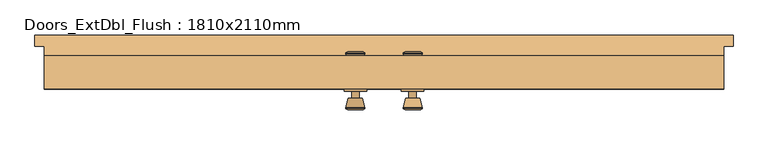
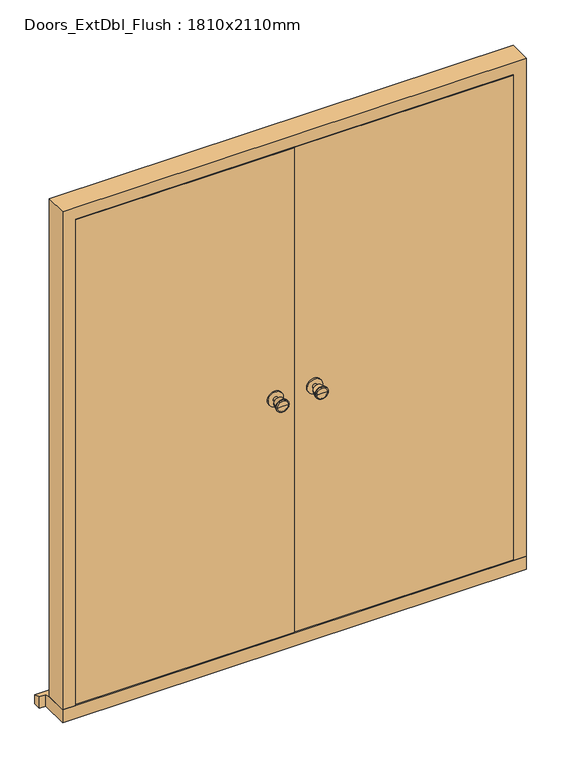
"""IFC4 building model written with IfcOpenShell, lengths in millimetres: door geometry, Doors_ExtDbl_Flush : 1810x2110mm."""

from ifc_helpers import new_model, si_unit, point, frame, frame_2d, origin, place, context, project, spatial, polyline, circle_curve, trimmed, segment, composite_curve, outline, extrude, faceted_brep, source, transform, mapped, element, save
from ifc_brep_helpers import plane_surface, cylinder_surface, revolved_surface, advanced_brep


def doors_extdbl_flush_1810x2110mm_0705243e(model_context):
    return source(origin(), model_context, "Body", "SolidModel", [
        advanced_brep(
        [(-76.5, -31.1, 1050.0), (-66.5, -31.1, 1050.0), (-86.5, -31.1, 1050.0), (-96.9758676, -80.1, 1050.0), (-56.0241324, -80.1, 1050.0), (-76.5, -80.1, 1050.0), (-101.5, -78.2721319, 1050.0), (-51.5, -78.2721319, 1050.0), (-101.5, -74.8084537, 1050.0), (-51.5, -74.8084537, 1050.0), (-95.136236, -50.1, 1050.0), (-57.863764, -50.1, 1050.0), (-86.5, -50.1, 1050.0), (-66.5, -50.1, 1050.0)],
        [
            (0, 1),
            (1, 2, circle_curve(frame((-76.5, -31.1, 1050.0), z_axis=(0.0, 1.0, 0.0), x_axis=(1.0, 0.0, 0.0)), 10.0)),
            (2, 0),
            (2, 1, circle_curve(frame((-76.5, -31.1, 1050.0), z_axis=(0.0, 1.0, 0.0), x_axis=(1.0, 0.0, 0.0)), 10.0)),
            (3, 4, circle_curve(frame((-76.5, -80.1, 1050.0), z_axis=(0.0, -1.0, 0.0), x_axis=(1.0, 0.0, 0.0)), 20.4758676)),
            (4, 5),
            (5, 3),
            (4, 3, circle_curve(frame((-76.5, -80.1, 1050.0), z_axis=(0.0, -1.0, 0.0), x_axis=(1.0, 0.0, 0.0)), 20.4758676)),
            (6, 7, circle_curve(frame((-76.5, -78.2721319, 1050.0), z_axis=(0.0, -1.0, 0.0), x_axis=(1.0, 0.0, 0.0)), 25.0)),
            (7, 4),
            (3, 6),
            (7, 6, circle_curve(frame((-76.5, -78.2721319, 1050.0), z_axis=(0.0, -1.0, 0.0), x_axis=(1.0, 0.0, 0.0)), 25.0)),
            (8, 9, circle_curve(frame((-76.5, -74.8084537, 1050.0), z_axis=(0.0, -1.0, 0.0), x_axis=(1.0, 0.0, 0.0)), 25.0)),
            (9, 7),
            (6, 8),
            (9, 8, circle_curve(frame((-76.5, -74.8084537, 1050.0), z_axis=(0.0, -1.0, 0.0), x_axis=(1.0, 0.0, 0.0)), 25.0)),
            (10, 11, circle_curve(frame((-76.5, -50.1, 1050.0), z_axis=(0.0, -1.0, 0.0), x_axis=(1.0, 0.0, 0.0)), 18.636236)),
            (11, 9),
            (8, 10),
            (11, 10, circle_curve(frame((-76.5, -50.1, 1050.0), z_axis=(0.0, -1.0, 0.0), x_axis=(1.0, 0.0, 0.0)), 18.636236)),
            (12, 13, circle_curve(frame((-76.5, -50.1, 1050.0), z_axis=(0.0, -1.0, 0.0), x_axis=(1.0, 0.0, 0.0)), 10.0)),
            (13, 11),
            (10, 12),
            (13, 12, circle_curve(frame((-76.5, -50.1, 1050.0), z_axis=(0.0, -1.0, 0.0), x_axis=(1.0, 0.0, 0.0)), 10.0)),
            (1, 13),
            (12, 2),
        ],
        [
            plane_surface(frame((-76.5, -31.1, 1050.0), z_axis=(0.0, 1.0, 0.0), x_axis=(1.0, 0.0, 0.0))),
            plane_surface(frame((-76.5, -80.1, 1050.0), z_axis=(0.0, -1.0, 0.0), x_axis=(1.0, 0.0, 0.0))),
            revolved_surface(polyline([(-56.0241324, -80.1, 1050.0), (-51.5, -78.2721319, 1050.0)]), (-76.5, -31.1, 1050.0), (0.0, 1.0, 0.0)),
            cylinder_surface(frame((-76.5, -31.1, 1050.0), z_axis=(0.0, 1.0, 0.0), x_axis=(1.0, 0.0, 0.0)), 25.0),
            revolved_surface(polyline([(-51.5, -74.8084537, 1050.0), (-57.863764, -50.1, 1050.0)]), (-76.5, -31.1, 1050.0), (0.0, 1.0, 0.0)),
            plane_surface(frame((-76.5, -50.1, 1050.0), z_axis=(0.0, 1.0, 0.0), x_axis=(1.0, 0.0, 0.0))),
            cylinder_surface(frame((-76.5, -31.1, 1050.0), z_axis=(0.0, 1.0, 0.0), x_axis=(1.0, 0.0, 0.0)), 10.0),
        ],
        [
            (0, [[1, 2, 3]]),
            (0, [[-3, 4, -1]]),
            (1, [[5, 6, 7]]),
            (1, [[8, -7, -6]]),
            (2, [[9, 10, -5, 11]]),
            (2, [[12, -11, -8, -10]]),
            (3, [[13, 14, -9, 15]]),
            (3, [[16, -15, -12, -14]]),
            (4, [[17, 18, -13, 19]]),
            (4, [[20, -19, -16, -18]]),
            (5, [[21, 22, -17, 23]]),
            (5, [[24, -23, -20, -22]]),
            (6, [[-2, 25, -21, 26]]),
            (6, [[-4, -26, -24, -25]]),
        ],
    ),
        extrude(outline(composite_curve([segment(trimmed(circle_curve(frame_2d((1050.0, -76.5)), 30.0), [point((1050.0, -46.5))], [point((1050.0, -106.5))], False, "CARTESIAN"), True, "CONTINUOUS"), segment(trimmed(circle_curve(frame_2d((1050.0, -76.5)), 30.0), [point((1050.0, -106.5))], [point((1050.0, -46.5))], False, "CARTESIAN"), True, "CONTINUOUS")], self_intersect=False)), frame((0.0, -31.1, 0.0), z_axis=(0.0, 1.0, 0.0), x_axis=(0.0, 0.0, 1.0)), (0.0, 0.0, 1.0), 6.0),
        advanced_brep(
        [(-76.5, 24.9, 1050.0), (-86.5, 24.9, 1050.0), (-66.5, 24.9, 1050.0), (-96.9758676, 73.9, 1050.0), (-76.5, 73.9, 1050.0), (-56.0241324, 73.9, 1050.0), (-101.5, 72.0721319, 1050.0), (-51.5, 72.0721319, 1050.0), (-101.5, 68.6084537, 1050.0), (-51.5, 68.6084537, 1050.0), (-95.136236, 43.9, 1050.0), (-57.863764, 43.9, 1050.0), (-86.5, 43.9, 1050.0), (-66.5, 43.9, 1050.0)],
        [
            (0, 1),
            (1, 2, circle_curve(frame((-76.5, 24.9, 1050.0), z_axis=(0.0, -1.0, 0.0), x_axis=(1.0, 0.0, 0.0)), 10.0)),
            (2, 0),
            (2, 1, circle_curve(frame((-76.5, 24.9, 1050.0), z_axis=(0.0, -1.0, 0.0), x_axis=(1.0, 0.0, 0.0)), 10.0)),
            (3, 4),
            (4, 5),
            (5, 3, circle_curve(frame((-76.5, 73.9, 1050.0), z_axis=(0.0, 1.0, 0.0), x_axis=(1.0, 0.0, 0.0)), 20.4758676)),
            (3, 5, circle_curve(frame((-76.5, 73.9, 1050.0), z_axis=(0.0, 1.0, 0.0), x_axis=(1.0, 0.0, 0.0)), 20.4758676)),
            (6, 3),
            (5, 7),
            (7, 6, circle_curve(frame((-76.5, 72.0721319, 1050.0), z_axis=(0.0, 1.0, 0.0), x_axis=(1.0, 0.0, 0.0)), 25.0)),
            (6, 7, circle_curve(frame((-76.5, 72.0721319, 1050.0), z_axis=(0.0, 1.0, 0.0), x_axis=(1.0, 0.0, 0.0)), 25.0)),
            (8, 6),
            (7, 9),
            (9, 8, circle_curve(frame((-76.5, 68.6084537, 1050.0), z_axis=(0.0, 1.0, 0.0), x_axis=(1.0, 0.0, 0.0)), 25.0)),
            (8, 9, circle_curve(frame((-76.5, 68.6084537, 1050.0), z_axis=(0.0, 1.0, 0.0), x_axis=(1.0, 0.0, 0.0)), 25.0)),
            (10, 8),
            (9, 11),
            (11, 10, circle_curve(frame((-76.5, 43.9, 1050.0), z_axis=(0.0, 1.0, 0.0), x_axis=(1.0, 0.0, 0.0)), 18.636236)),
            (10, 11, circle_curve(frame((-76.5, 43.9, 1050.0), z_axis=(0.0, 1.0, 0.0), x_axis=(1.0, 0.0, 0.0)), 18.636236)),
            (12, 10),
            (11, 13),
            (13, 12, circle_curve(frame((-76.5, 43.9, 1050.0), z_axis=(0.0, 1.0, 0.0), x_axis=(1.0, 0.0, 0.0)), 10.0)),
            (12, 13, circle_curve(frame((-76.5, 43.9, 1050.0), z_axis=(0.0, 1.0, 0.0), x_axis=(1.0, 0.0, 0.0)), 10.0)),
            (1, 12),
            (13, 2),
        ],
        [
            plane_surface(frame((-76.5, 24.9, 1050.0), z_axis=(0.0, -1.0, 0.0), x_axis=(1.0, 0.0, 0.0))),
            plane_surface(frame((-76.5, 73.9, 1050.0), z_axis=(0.0, 1.0, 0.0), x_axis=(1.0, 0.0, 0.0))),
            revolved_surface(polyline([(-56.0241324, 73.9, 1050.0), (-51.5, 72.0721319, 1050.0)]), (-76.5, 24.9, 1050.0), (0.0, -1.0, 0.0)),
            cylinder_surface(frame((-76.5, 24.9, 1050.0), z_axis=(0.0, -1.0, 0.0), x_axis=(1.0, 0.0, 0.0)), 25.0),
            revolved_surface(polyline([(-51.5, 68.6084537, 1050.0), (-57.863764, 43.9, 1050.0)]), (-76.5, 24.9, 1050.0), (0.0, -1.0, 0.0)),
            plane_surface(frame((-76.5, 43.9, 1050.0), z_axis=(0.0, -1.0, 0.0), x_axis=(1.0, 0.0, 0.0))),
            cylinder_surface(frame((-76.5, 24.9, 1050.0), z_axis=(0.0, -1.0, 0.0), x_axis=(1.0, 0.0, 0.0)), 10.0),
        ],
        [
            (0, [[1, 2, 3]]),
            (0, [[-3, 4, -1]]),
            (1, [[5, 6, 7]]),
            (1, [[-6, -5, 8]]),
            (2, [[9, -7, 10, 11]]),
            (2, [[-10, -8, -9, 12]]),
            (3, [[13, -11, 14, 15]]),
            (3, [[-14, -12, -13, 16]]),
            (4, [[17, -15, 18, 19]]),
            (4, [[-18, -16, -17, 20]]),
            (5, [[21, -19, 22, 23]]),
            (5, [[-22, -20, -21, 24]]),
            (6, [[25, -23, 26, -2]]),
            (6, [[-26, -24, -25, -4]]),
        ],
    ),
        extrude(outline(composite_curve([segment(trimmed(circle_curve(frame_2d((1050.0, -76.5)), 30.0), [point((1050.0, -46.5))], [point((1050.0, -106.5))], False, "CARTESIAN"), True, "CONTINUOUS"), segment(trimmed(circle_curve(frame_2d((1050.0, -76.5)), 30.0), [point((1050.0, -106.5))], [point((1050.0, -46.5))], False, "CARTESIAN"), True, "CONTINUOUS")], self_intersect=False)), frame((0.0, 18.9, 0.0), z_axis=(0.0, 1.0, 0.0), x_axis=(0.0, 0.0, 1.0)), (0.0, 0.0, 1.0), 6.0),
        advanced_brep(
        [(76.5, -31.1, 1050.0), (86.5, -31.1, 1050.0), (66.5, -31.1, 1050.0), (96.9758676, -80.1, 1050.0), (76.5, -80.1, 1050.0), (56.0241324, -80.1, 1050.0), (101.5, -78.2721319, 1050.0), (51.5, -78.2721319, 1050.0), (101.5, -74.8084537, 1050.0), (51.5, -74.8084537, 1050.0), (95.136236, -50.1, 1050.0), (57.863764, -50.1, 1050.0), (86.5, -50.1, 1050.0), (66.5, -50.1, 1050.0)],
        [
            (0, 1),
            (1, 2, circle_curve(frame((76.5, -31.1, 1050.0), z_axis=(0.0, 1.0, 0.0), x_axis=(-1.0, 0.0, 0.0)), 10.0)),
            (2, 0),
            (2, 1, circle_curve(frame((76.5, -31.1, 1050.0), z_axis=(0.0, 1.0, 0.0), x_axis=(-1.0, 0.0, 0.0)), 10.0)),
            (3, 4),
            (4, 5),
            (5, 3, circle_curve(frame((76.5, -80.1, 1050.0), z_axis=(0.0, -1.0, 0.0), x_axis=(-1.0, 0.0, 0.0)), 20.4758676)),
            (3, 5, circle_curve(frame((76.5, -80.1, 1050.0), z_axis=(0.0, -1.0, 0.0), x_axis=(-1.0, 0.0, 0.0)), 20.4758676)),
            (6, 3),
            (5, 7),
            (7, 6, circle_curve(frame((76.5, -78.2721319, 1050.0), z_axis=(0.0, -1.0, 0.0), x_axis=(-1.0, 0.0, 0.0)), 25.0)),
            (6, 7, circle_curve(frame((76.5, -78.2721319, 1050.0), z_axis=(0.0, -1.0, 0.0), x_axis=(-1.0, 0.0, 0.0)), 25.0)),
            (8, 6),
            (7, 9),
            (9, 8, circle_curve(frame((76.5, -74.8084537, 1050.0), z_axis=(0.0, -1.0, 0.0), x_axis=(-1.0, 0.0, 0.0)), 25.0)),
            (8, 9, circle_curve(frame((76.5, -74.8084537, 1050.0), z_axis=(0.0, -1.0, 0.0), x_axis=(-1.0, 0.0, 0.0)), 25.0)),
            (10, 8),
            (9, 11),
            (11, 10, circle_curve(frame((76.5, -50.1, 1050.0), z_axis=(0.0, -1.0, 0.0), x_axis=(-1.0, 0.0, 0.0)), 18.636236)),
            (10, 11, circle_curve(frame((76.5, -50.1, 1050.0), z_axis=(0.0, -1.0, 0.0), x_axis=(-1.0, 0.0, 0.0)), 18.636236)),
            (12, 10),
            (11, 13),
            (13, 12, circle_curve(frame((76.5, -50.1, 1050.0), z_axis=(0.0, -1.0, 0.0), x_axis=(-1.0, 0.0, 0.0)), 10.0)),
            (12, 13, circle_curve(frame((76.5, -50.1, 1050.0), z_axis=(0.0, -1.0, 0.0), x_axis=(-1.0, 0.0, 0.0)), 10.0)),
            (1, 12),
            (13, 2),
        ],
        [
            plane_surface(frame((76.5, -31.1, 1050.0), z_axis=(0.0, 1.0, 0.0), x_axis=(-1.0, 0.0, 0.0))),
            plane_surface(frame((76.5, -80.1, 1050.0), z_axis=(0.0, -1.0, 0.0), x_axis=(-1.0, 0.0, 0.0))),
            revolved_surface(polyline([(56.0241324, -80.1, 1050.0), (51.5, -78.2721319, 1050.0)]), (76.5, -31.1, 1050.0), (0.0, 1.0, 0.0)),
            cylinder_surface(frame((76.5, -31.1, 1050.0), z_axis=(0.0, 1.0, 0.0), x_axis=(-1.0, 0.0, 0.0)), 25.0),
            revolved_surface(polyline([(51.5, -74.8084537, 1050.0), (57.863764, -50.1, 1050.0)]), (76.5, -31.1, 1050.0), (0.0, 1.0, 0.0)),
            plane_surface(frame((76.5, -50.1, 1050.0), z_axis=(0.0, 1.0, 0.0), x_axis=(-1.0, 0.0, 0.0))),
            cylinder_surface(frame((76.5, -31.1, 1050.0), z_axis=(0.0, 1.0, 0.0), x_axis=(-1.0, 0.0, 0.0)), 10.0),
        ],
        [
            (0, [[1, 2, 3]]),
            (0, [[-3, 4, -1]]),
            (1, [[5, 6, 7]]),
            (1, [[-6, -5, 8]]),
            (2, [[9, -7, 10, 11]]),
            (2, [[-10, -8, -9, 12]]),
            (3, [[13, -11, 14, 15]]),
            (3, [[-14, -12, -13, 16]]),
            (4, [[17, -15, 18, 19]]),
            (4, [[-18, -16, -17, 20]]),
            (5, [[21, -19, 22, 23]]),
            (5, [[-22, -20, -21, 24]]),
            (6, [[25, -23, 26, -2]]),
            (6, [[-26, -24, -25, -4]]),
        ],
    ),
        extrude(outline(composite_curve([segment(trimmed(circle_curve(frame_2d((1050.0, 76.5)), 30.0), [point((1050.0, 46.5))], [point((1050.0, 106.5))], False, "CARTESIAN"), True, "CONTINUOUS"), segment(trimmed(circle_curve(frame_2d((1050.0, 76.5)), 30.0), [point((1050.0, 106.5))], [point((1050.0, 46.5))], False, "CARTESIAN"), True, "CONTINUOUS")], self_intersect=False)), frame((0.0, -31.1, 0.0), z_axis=(0.0, 1.0, 0.0), x_axis=(0.0, 0.0, 1.0)), (0.0, 0.0, 1.0), 6.0),
        advanced_brep(
        [(76.5, 24.9, 1050.0), (66.5, 24.9, 1050.0), (86.5, 24.9, 1050.0), (96.9758676, 73.9, 1050.0), (56.0241324, 73.9, 1050.0), (76.5, 73.9, 1050.0), (101.5, 72.0721319, 1050.0), (51.5, 72.0721319, 1050.0), (101.5, 68.6084537, 1050.0), (51.5, 68.6084537, 1050.0), (95.136236, 43.9, 1050.0), (57.863764, 43.9, 1050.0), (86.5, 43.9, 1050.0), (66.5, 43.9, 1050.0)],
        [
            (0, 1),
            (1, 2, circle_curve(frame((76.5, 24.9, 1050.0), z_axis=(0.0, -1.0, 0.0), x_axis=(-1.0, 0.0, 0.0)), 10.0)),
            (2, 0),
            (2, 1, circle_curve(frame((76.5, 24.9, 1050.0), z_axis=(0.0, -1.0, 0.0), x_axis=(-1.0, 0.0, 0.0)), 10.0)),
            (3, 4, circle_curve(frame((76.5, 73.9, 1050.0), z_axis=(0.0, 1.0, 0.0), x_axis=(-1.0, 0.0, 0.0)), 20.4758676)),
            (4, 5),
            (5, 3),
            (4, 3, circle_curve(frame((76.5, 73.9, 1050.0), z_axis=(0.0, 1.0, 0.0), x_axis=(-1.0, 0.0, 0.0)), 20.4758676)),
            (6, 7, circle_curve(frame((76.5, 72.0721319, 1050.0), z_axis=(0.0, 1.0, 0.0), x_axis=(-1.0, 0.0, 0.0)), 25.0)),
            (7, 4),
            (3, 6),
            (7, 6, circle_curve(frame((76.5, 72.0721319, 1050.0), z_axis=(0.0, 1.0, 0.0), x_axis=(-1.0, 0.0, 0.0)), 25.0)),
            (8, 9, circle_curve(frame((76.5, 68.6084537, 1050.0), z_axis=(0.0, 1.0, 0.0), x_axis=(-1.0, 0.0, 0.0)), 25.0)),
            (9, 7),
            (6, 8),
            (9, 8, circle_curve(frame((76.5, 68.6084537, 1050.0), z_axis=(0.0, 1.0, 0.0), x_axis=(-1.0, 0.0, 0.0)), 25.0)),
            (10, 11, circle_curve(frame((76.5, 43.9, 1050.0), z_axis=(0.0, 1.0, 0.0), x_axis=(-1.0, 0.0, 0.0)), 18.636236)),
            (11, 9),
            (8, 10),
            (11, 10, circle_curve(frame((76.5, 43.9, 1050.0), z_axis=(0.0, 1.0, 0.0), x_axis=(-1.0, 0.0, 0.0)), 18.636236)),
            (12, 13, circle_curve(frame((76.5, 43.9, 1050.0), z_axis=(0.0, 1.0, 0.0), x_axis=(-1.0, 0.0, 0.0)), 10.0)),
            (13, 11),
            (10, 12),
            (13, 12, circle_curve(frame((76.5, 43.9, 1050.0), z_axis=(0.0, 1.0, 0.0), x_axis=(-1.0, 0.0, 0.0)), 10.0)),
            (1, 13),
            (12, 2),
        ],
        [
            plane_surface(frame((76.5, 24.9, 1050.0), z_axis=(0.0, -1.0, 0.0), x_axis=(-1.0, 0.0, 0.0))),
            plane_surface(frame((76.5, 73.9, 1050.0), z_axis=(0.0, 1.0, 0.0), x_axis=(-1.0, 0.0, 0.0))),
            revolved_surface(polyline([(56.0241324, 73.9, 1050.0), (51.5, 72.0721319, 1050.0)]), (76.5, 24.9, 1050.0), (0.0, -1.0, 0.0)),
            cylinder_surface(frame((76.5, 24.9, 1050.0), z_axis=(0.0, -1.0, 0.0), x_axis=(-1.0, 0.0, 0.0)), 25.0),
            revolved_surface(polyline([(51.5, 68.6084537, 1050.0), (57.863764, 43.9, 1050.0)]), (76.5, 24.9, 1050.0), (0.0, -1.0, 0.0)),
            plane_surface(frame((76.5, 43.9, 1050.0), z_axis=(0.0, -1.0, 0.0), x_axis=(-1.0, 0.0, 0.0))),
            cylinder_surface(frame((76.5, 24.9, 1050.0), z_axis=(0.0, -1.0, 0.0), x_axis=(-1.0, 0.0, 0.0)), 10.0),
        ],
        [
            (0, [[1, 2, 3]]),
            (0, [[-3, 4, -1]]),
            (1, [[5, 6, 7]]),
            (1, [[8, -7, -6]]),
            (2, [[9, 10, -5, 11]]),
            (2, [[12, -11, -8, -10]]),
            (3, [[13, 14, -9, 15]]),
            (3, [[16, -15, -12, -14]]),
            (4, [[17, 18, -13, 19]]),
            (4, [[20, -19, -16, -18]]),
            (5, [[21, 22, -17, 23]]),
            (5, [[24, -23, -20, -22]]),
            (6, [[-2, 25, -21, 26]]),
            (6, [[-4, -26, -24, -25]]),
        ],
    ),
        extrude(outline(composite_curve([segment(trimmed(circle_curve(frame_2d((1050.0, 76.5)), 30.0), [point((1050.0, 46.5))], [point((1050.0, 106.5))], False, "CARTESIAN"), True, "CONTINUOUS"), segment(trimmed(circle_curve(frame_2d((1050.0, 76.5)), 30.0), [point((1050.0, 106.5))], [point((1050.0, 46.5))], False, "CARTESIAN"), True, "CONTINUOUS")], self_intersect=False)), frame((0.0, 18.9, 0.0), z_axis=(0.0, 1.0, 0.0), x_axis=(0.0, 0.0, 1.0)), (0.0, 0.0, 1.0), 6.0),
        faceted_brep([(834.5, 63.9, 54.5), (905.0, 63.9, 54.5), (905.0, -25.1, 54.5), (856.5, -25.1, 54.5), (856.5, 21.9, 54.5), (834.5, 21.9, 54.5), (834.5, 63.9, 2039.5), (-834.5, 63.9, 2039.5), (-834.5, 63.9, 54.5), (-905.0, 63.9, 54.5), (-905.0, 63.9, 2110.0), (905.0, 63.9, 2110.0), (905.0, -25.1, 2110.0), (-905.0, -25.1, 2110.0), (-905.0, -25.1, 54.5), (-856.5, -25.1, 54.5), (-856.5, -25.1, 2061.5), (856.5, -25.1, 2061.5), (856.5, 21.9, 2061.5), (-856.5, 21.9, 2061.5), (-856.5, 21.9, 54.5), (-834.5, 21.9, 54.5), (-834.5, 21.9, 2039.5), (834.5, 21.9, 2039.5)], [[[0, 1, 2, 3, 4, 5]], [[1, 0, 6, 7, 8, 9, 10, 11]], [[2, 1, 11, 12]], [[3, 2, 12, 13, 14, 15, 16, 17]], [[4, 3, 17, 18]], [[5, 4, 18, 19, 20, 21, 22, 23]], [[0, 5, 23, 6]], [[12, 11, 10, 13]], [[18, 17, 16, 19]], [[6, 23, 22, 7]], [[8, 21, 20, 15, 14, 9]], [[13, 10, 9, 14]], [[19, 16, 15, 20]], [[7, 22, 21, 8]]]),
        faceted_brep([(930.0, 118.9, 0.0), (930.0, 118.9, 38.5947221), (930.0, 88.9, 47.2703282), (930.0, 88.9, 0.0), (-930.0, 118.9, 38.5947221), (-930.0, 118.9, 0.0), (-930.0, 88.9, 0.0), (-930.0, 88.9, 47.2703282), (905.0, 88.9, 0.0), (905.0, -25.1, 0.0), (-905.0, -25.1, 0.0), (-905.0, 88.9, 0.0), (-905.0, 88.9, 47.2703282), (-905.0, 63.9, 54.5), (905.0, 63.9, 54.5), (905.0, 88.9, 47.2703282), (-905.0, -25.1, 54.5), (905.0, -25.1, 54.5)], [[[0, 1, 2, 3]], [[4, 5, 6, 7]], [[5, 0, 3, 8, 9, 10, 11, 6]], [[1, 0, 5, 4]], [[1, 4, 7, 12, 13, 14, 15, 2]], [[13, 16, 17, 14]], [[16, 10, 9, 17]], [[12, 11, 10, 16, 13]], [[11, 12, 7, 6]], [[8, 15, 14, 17, 9]], [[15, 8, 3, 2]]]),
        extrude(outline(polyline([(853.5, -25.1), (1.5, -25.1), (1.5, 18.9), (853.5, 18.9), (853.5, -25.1)])), frame((0.0, 0.0, 58.5), z_axis=(0.0, 0.0, 1.0), x_axis=(1.0, 0.0, 0.0)), (0.0, 0.0, 1.0), 2000.0),
        extrude(outline(polyline([(-1.5, -25.1), (-853.5, -25.1), (-853.5, 18.9), (-1.5, 18.9), (-1.5, -25.1)])), frame((0.0, 0.0, 58.5), z_axis=(0.0, 0.0, 1.0), x_axis=(1.0, 0.0, 0.0)), (0.0, 0.0, 1.0), 2000.0),
    ])


if __name__ == "__main__":
    model = new_model("IFC4")
    model_context = context("Model", 3, world=origin())
    ifc_project = project(units=[si_unit("LENGTHUNIT", "METRE", prefix="MILLI")], contexts=[model_context])
    site = spatial("IfcSite", under=ifc_project)
    building = spatial("IfcBuilding", under=site)
    placement = place(None, origin())
    doors_extdbl_flush_1810x2110mm_shape = doors_extdbl_flush_1810x2110mm_0705243e(model_context)
    element("IfcDoor", 1, ObjectType="Doors_ExtDbl_Flush : 1810x2110mm", at=placement, inside=building, context=model_context, shape_type="MappedRepresentation", body=[
        mapped(doors_extdbl_flush_1810x2110mm_shape, transform((0.0, 0.0, 0.0), x_axis=(1.0, 0.0, 0.0), y_axis=(0.0, 1.0, 0.0), z_axis=(0.0, 0.0, 1.0))),
    ])
    save(model, "model.ifc")

# Revit data of these elements
# Type "Doors_ExtDbl_Flush : 1810x2110mm"
#   Type Mark = "44"
#   Type Comments = "External Double"
#   Operation = "DoubleDoorSingleSwing"
#   Keynote = "L20"
#   Analytic Construction = "Metal"
#   Wrap Layers (Ext) from Ext = 0' - 4.03543"
#   Wrap Layers (Int) from Ext = 0' - 6.98819"
#   Thickness = 0' - 1.73228"
#   Rough Width = 5' - 11.25984"
#   Rough Height = 6' - 11.07087"
#   O/A Frame Width = 0' - 2.51969"
#   Heat Transfer Coefficient (U) = 3.7021 W/(m²·K)
#   Handle Z Distance = 3' - 5.33858"
#   FrameWidth = 0' - 1.65354"
#   FrameOffset - External = 0' - 0.98425"
#   FrameDepth = 0' - 3.50394"
#   Door Panel Width = 2' - 9.54331"
#   Door Panel Thickness = 0' - 1.73228"
#   Door Panel Height = 6' - 6.74016"
#   Cill Thickness = 0' - 2.14567"
#   Cill Projection = 0' - 1.1811"
#   Handle X Distance = 0' - 2.95276"
#   Height = 6' - 11.07087"
#   Structural Tolerance = 0' - 0.25591"
#   Tolerance = 0' - 0.11811"
#   Undercut = 0' - 0.15748"
#   Width = 5' - 11.25984"
#   Cill Extension = 0' - 0.98425"
#   Cavity Closer Width = 0' - 1.9685"
#   Cavity Closer Offset from Ext = 0' - 4.03543"
#   Cavity Closer Depth = 0' - 3.34646"
#   Define Thermal Properties by = 0
#   Vis - Ironmongery = yes
#   Vis - Cavity Closers = yes
#   Function = 1
#   Material Door = Door - Panel
#   Material Frame = Door - Frame/Mullion
#   Material Ironmongery = Door - Handle
#   Visual Light Transmittance = 0
#   Thermal Resistance (R) = 0
#   Solar Heat Gain Coefficient = 0
#   Wall Closure = (empty or 0)
# Element 1 (IfcDoor, "Doors_ExtDbl_Flush : 1810x2110mm")
#   Materials on its faces: "Door - Handle", "Door - Frame/Mullion", "Door - Panel"
# Materials
#   "Door - Panel": class "Wood", colour RGB 210 159 95, transparency 0, Keynote = "L20", Cost = 0
#   "Door - Frame/Mullion": class "Wood", colour RGB 212 179 113, transparency 0, Keynote = "L20", Cost = 0
#   "Door - Handle": colour RGB 0 0 0, transparency 0, Keynote = "P21", Cost = 0
